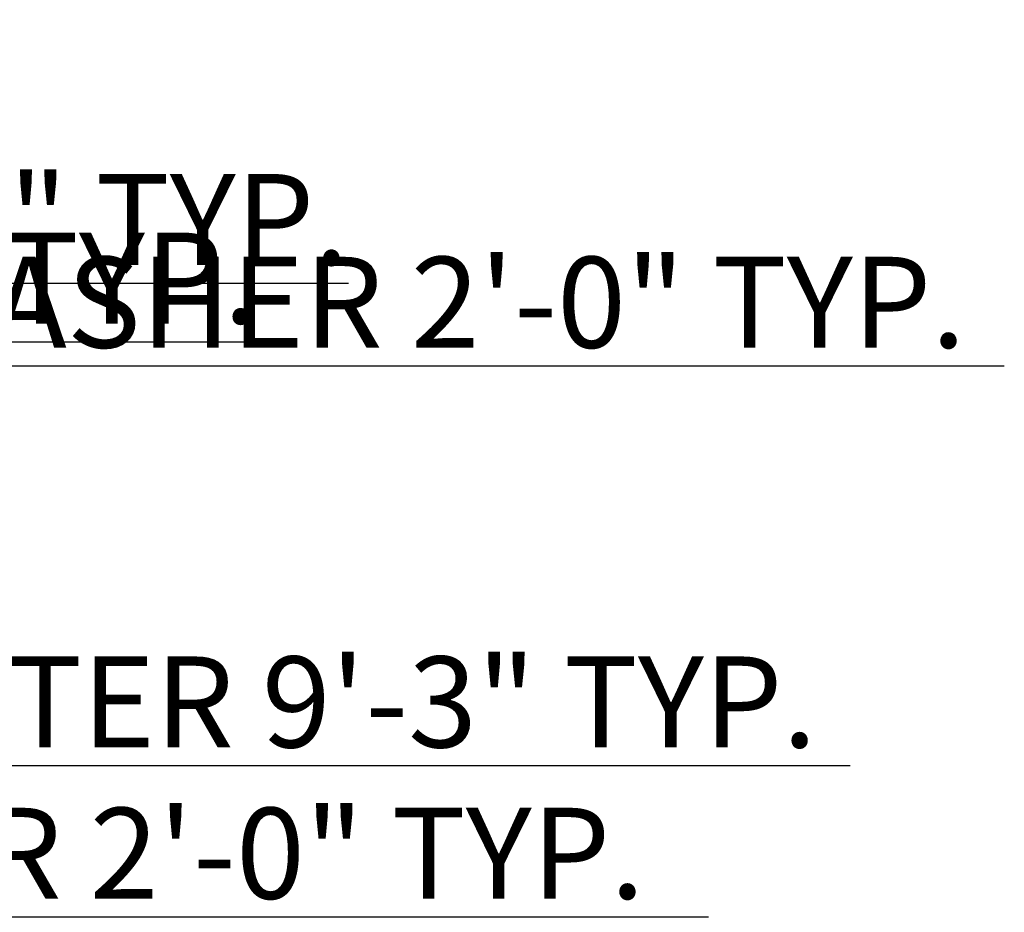
# Model space of a CAD drawing. Units: inches. Extents: x 375 to 1122, y 27 to 1069.
# Tile 155 of 155: x 992 to 1122, y 872 to 989. Entities that reach past the tile are written whole.
import ezdxf

# ---------------------------------------------------------------- set-up
doc = ezdxf.new("R2010")
doc.units = ezdxf.units.IN
doc.layers.add('A-ANNO-DIMS', color=2, linetype='Continuous', lineweight=18)
doc.styles.get("Standard").update_dxf_attribs({"font": 'arial.ttf'})
doc.dimstyles.new('ISO-25', dxfattribs={"dimtxt": 12, "dimasz": 2.5, "dimexe": 1.5, "dimexo": 1.5, "dimtad": 1, "dimdec": 1, "dimlunit": 3, "dimtxsty": 'Standard', "dimblk": 'ARCHTICK', "dimcen": 2.5, "dimadec": 0, "dimazin": 0, "dimtfac": 1, "dimtdec": 1, "dimtmove": 0, "dimatfit": 3, "dimfxl": 1.5, "dimfxlon": 1, "dimarcsym": 0})

# ---------------------------------------------------------------- blocks, each defined once
blk = doc.blocks.new('_ArchTick')
at = {"color": 0, "linetype": 'ByBlock', "const_width": 0.15}
blk.add_lwpolyline([(-0.5, -0.5), (0.5, 0.5)], dxfattribs=at)
blk = doc.blocks.new('*D61')
at = {"layer": 'A-ANNO-DIMS', "color": 0, "lineweight": -2, "transparency": 16777216}
for p, q in [((845.01, 872.43), (845.01, 869.43)), ((869.01, 872.43), (869.01, 869.43)), ((845.01, 870.93), (869.01, 870.93)), ((869.01, 870.93), (1083.13, 870.93))]:
    blk.add_line(p, q, dxfattribs=at)
at = {"layer": 'Defpoints', "color": 0, "transparency": 16777216}
for p in [(845.01, 874.53), (869.01, 874.53), (869.01, 870.93)]:
    blk.add_point(p, dxfattribs=at)
at = {"layer": 'A-ANNO-DIMS', "color": 0, "lineweight": -2, "transparency": 16777216, "xscale": 2.5, "yscale": 2.5, "zscale": 2.5, "rotation": 180}
blk.add_blockref('_ArchTick', (845.01, 870.93), dxfattribs=at)
at = {"layer": 'A-ANNO-DIMS', "color": 0, "lineweight": -2, "transparency": 16777216, "xscale": 2.5, "yscale": 2.5, "zscale": 2.5}
blk.add_blockref('_ArchTick', (869.01, 870.93), dxfattribs=at)
at = {"layer": 'A-ANNO-DIMS', "color": 0, "transparency": 16777216, "insert": (977.32, 877.76), "char_height": 12, "attachment_point": 5}
blk.add_mtext('REFRIGERATOR 2\'-0" TYP.', dxfattribs=at)
blk = doc.blocks.new('*D64')
at = {"layer": 'A-ANNO-DIMS', "color": 0, "lineweight": -2, "transparency": 16777216}
for p, q in [((900.04, 953.03), (900.04, 956.03)), ((922.58, 953.03), (922.58, 956.03)), ((900.04, 954.53), (922.58, 954.53)), ((922.58, 954.53), (1035.63, 954.53))]:
    blk.add_line(p, q, dxfattribs=at)
at = {"layer": 'Defpoints', "color": 0, "transparency": 16777216}
for p in [(922.58, 954.53), (900.04, 948.53), (922.58, 948.53)]:
    blk.add_point(p, dxfattribs=at)
at = {"layer": 'A-ANNO-DIMS', "color": 0, "lineweight": -2, "transparency": 16777216, "xscale": 2.5, "yscale": 2.5, "zscale": 2.5, "rotation": 180}
blk.add_blockref('_ArchTick', (900.04, 954.53), dxfattribs=at)
at = {"layer": 'A-ANNO-DIMS', "color": 0, "lineweight": -2, "transparency": 16777216, "xscale": 2.5, "yscale": 2.5, "zscale": 2.5}
blk.add_blockref('_ArchTick', (922.58, 954.53), dxfattribs=at)
at = {"layer": 'A-ANNO-DIMS', "color": 0, "transparency": 16777216, "insert": (980.36, 961.36), "char_height": 12, "attachment_point": 5}
blk.add_mtext('1\'-10 1/2" TYP.', dxfattribs=at)
blk = doc.blocks.new('*D65')
at = {"layer": 'A-ANNO-DIMS', "color": 0, "lineweight": -2, "transparency": 16777216}
for p, q in [((942.55, 945.11), (942.55, 942.11)), ((966.55, 945.11), (966.55, 942.11)), ((942.55, 943.61), (966.55, 943.61)), ((966.55, 943.61), (1122.17, 943.61))]:
    blk.add_line(p, q, dxfattribs=at)
at = {"layer": 'Defpoints', "color": 0, "transparency": 16777216}
for p in [(942.55, 947.21), (966.55, 947.21), (966.55, 943.61)]:
    blk.add_point(p, dxfattribs=at)
at = {"layer": 'A-ANNO-DIMS', "color": 0, "lineweight": -2, "transparency": 16777216, "xscale": 2.5, "yscale": 2.5, "zscale": 2.5, "rotation": 180}
blk.add_blockref('_ArchTick', (942.55, 943.61), dxfattribs=at)
at = {"layer": 'A-ANNO-DIMS', "color": 0, "lineweight": -2, "transparency": 16777216, "xscale": 2.5, "yscale": 2.5, "zscale": 2.5}
blk.add_blockref('_ArchTick', (966.55, 943.61), dxfattribs=at)
at = {"layer": 'A-ANNO-DIMS', "color": 0, "transparency": 16777216, "insert": (1045.61, 950.44), "char_height": 12, "attachment_point": 5}
blk.add_mtext('WASHER 2\'-0" TYP.', dxfattribs=at)
blk = doc.blocks.new('*D67')
at = {"layer": 'A-ANNO-DIMS', "color": 0, "lineweight": -2, "transparency": 16777216}
for p, q in [((819.23, 948.29), (819.23, 945.29)), ((853.33, 948.29), (853.33, 945.29)), ((819.23, 946.79), (853.33, 946.79)), ((853.33, 946.79), (1027.89, 946.79))]:
    blk.add_line(p, q, dxfattribs=at)
at = {"layer": 'Defpoints', "color": 0, "transparency": 16777216}
for p in [(819.23, 951.91), (853.33, 951.91), (853.33, 946.79)]:
    blk.add_point(p, dxfattribs=at)
at = {"layer": 'A-ANNO-DIMS', "color": 0, "lineweight": -2, "transparency": 16777216, "xscale": 2.5, "yscale": 2.5, "zscale": 2.5, "rotation": 180}
blk.add_blockref('_ArchTick', (819.23, 946.79), dxfattribs=at)
at = {"layer": 'A-ANNO-DIMS', "color": 0, "lineweight": -2, "transparency": 16777216, "xscale": 2.5, "yscale": 2.5, "zscale": 2.5}
blk.add_blockref('_ArchTick', (853.33, 946.79), dxfattribs=at)
at = {"layer": 'A-ANNO-DIMS', "color": 0, "transparency": 16777216, "insert": (941.86, 953.63), "char_height": 12, "attachment_point": 5}
blk.add_mtext('COOKTOP 2\'-10" TYP.', dxfattribs=at)
blk = doc.blocks.new('*D77')
at = {"layer": 'A-ANNO-DIMS', "color": 0, "lineweight": -2, "transparency": 16777216}
for p, q in [((812.01, 892.38), (812.01, 889.38)), ((923.01, 892.38), (923.01, 889.38)), ((812.01, 890.88), (923.01, 890.88)), ((923.01, 890.88), (1101.82, 890.88))]:
    blk.add_line(p, q, dxfattribs=at)
at = {"layer": 'Defpoints', "color": 0, "transparency": 16777216}
for p in [(812.01, 907.53), (923.01, 907.53), (923.01, 890.88)]:
    blk.add_point(p, dxfattribs=at)
at = {"layer": 'A-ANNO-DIMS', "color": 0, "lineweight": -2, "transparency": 16777216, "xscale": 2.5, "yscale": 2.5, "zscale": 2.5, "rotation": 180}
blk.add_blockref('_ArchTick', (812.01, 890.88), dxfattribs=at)
at = {"layer": 'A-ANNO-DIMS', "color": 0, "lineweight": -2, "transparency": 16777216, "xscale": 2.5, "yscale": 2.5, "zscale": 2.5}
blk.add_blockref('_ArchTick', (923.01, 890.88), dxfattribs=at)
at = {"layer": 'A-ANNO-DIMS', "color": 0, "transparency": 16777216, "insert": (1013.66, 897.72), "char_height": 12, "attachment_point": 5}
blk.add_mtext('L-COUNTER 9\'-3" TYP.', dxfattribs=at)

msp = doc.modelspace()

# ---------------------------------------------------------------- dimensions: what is measured, and where the dimension line sits
at = {"layer": 'A-ANNO-DIMS'}
for base, p1, p2, text, picture, middle in [((922.58, 954.53), (900.04, 948.53), (922.58, 948.53), '<> TYP.', '*D64', (980.36, 961.36)), ((853.33, 946.79), (819.23, 951.91), (853.33, 951.91), 'COOKTOP <> TYP.', '*D67', (941.86, 953.63)), ((966.55, 943.61), (942.55, 947.21), (966.55, 947.21), 'WASHER <> TYP.', '*D65', (1045.61, 950.44)), ((923.01, 890.88), (812.01, 907.53), (923.01, 907.53), 'L-COUNTER <> TYP.', '*D77', (1013.66, 897.72)), ((869.01, 870.93), (845.01, 874.53), (869.01, 874.53), 'REFRIGERATOR <> TYP.', '*D61', (977.32, 877.76))]:
    dim = msp.add_linear_dim(base=base, p1=p1, p2=p2, text=text, dimstyle='ISO-25', override={"dimdec": 1, "dimlfac": 1, "dimrnd": 0, "dimzin": 1, "dimdsep": 46, "dimlunit": 4, "dimfrac": 2}, dxfattribs=at)
    dim.commit()
    dim.dimension.update_dxf_attribs({"geometry": picture, "text_midpoint": middle})

doc.saveas('drawing.dxf')
